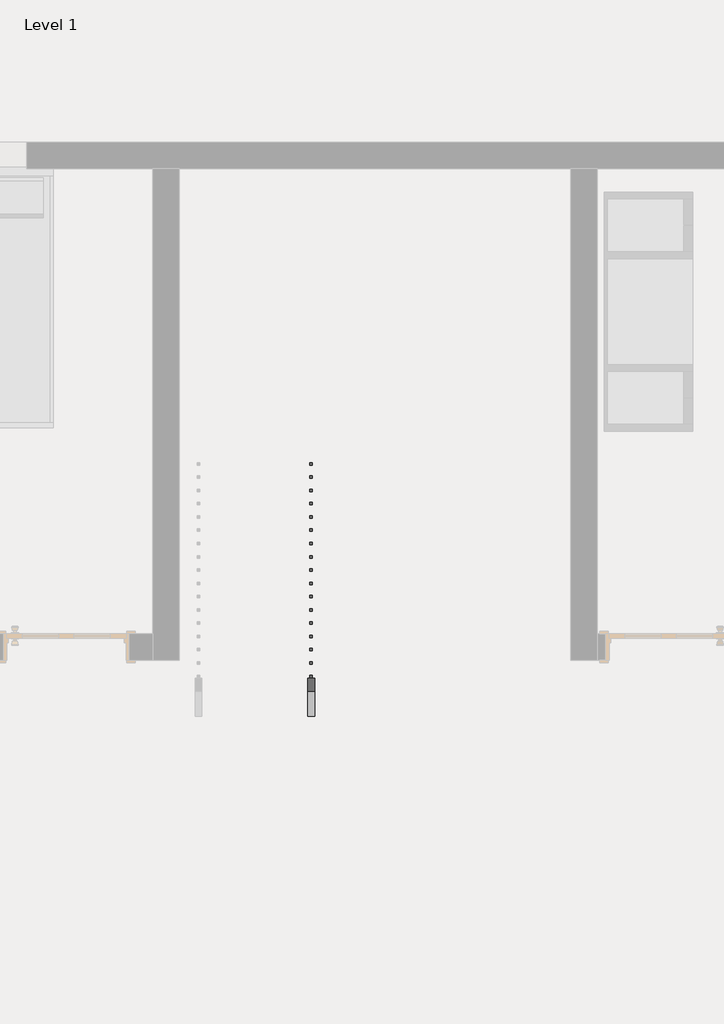
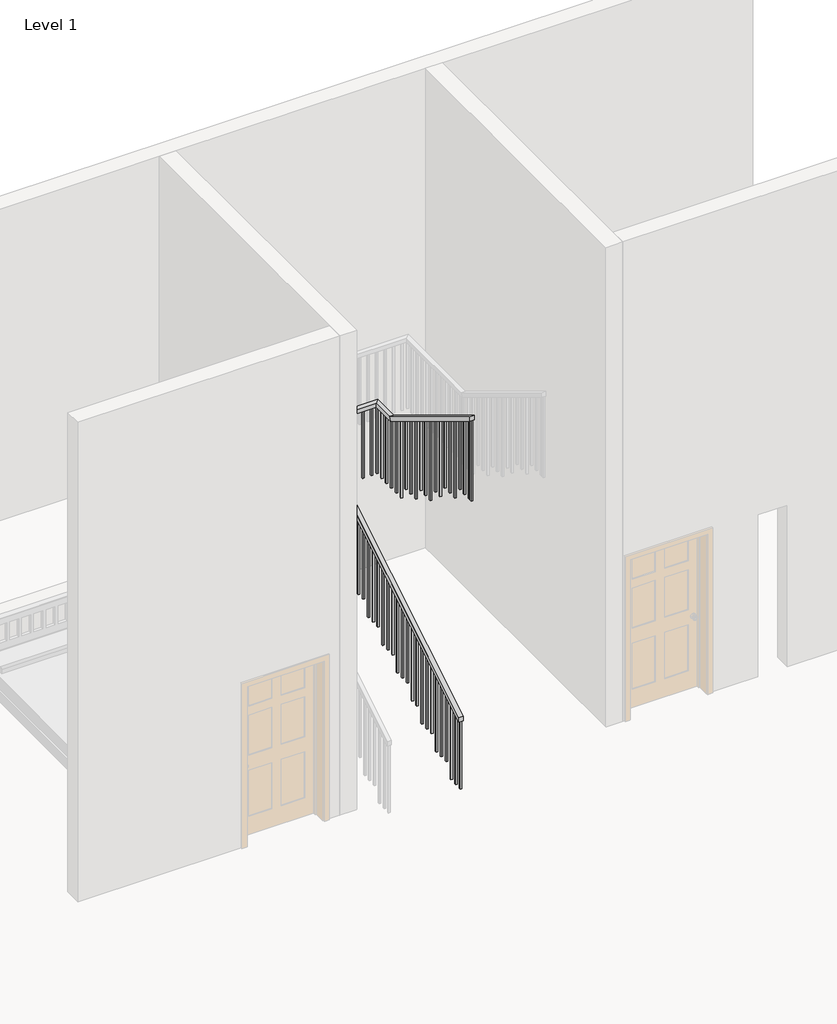
# One storey, part 2 of 3: 1 railing.
"""IFC4 building model written with IfcOpenShell, lengths in millimetres."""

from ifc_helpers import new_model, si_unit, frame, origin, place, context, project, spatial, polyline, outline, extrude, faceted_brep, element, save

model = new_model("IFC4")

# Units and contexts
model_context = context("Model", 3, world=origin())
ifc_project = project(units=[si_unit("LENGTHUNIT", "METRE", prefix="MILLI")], contexts=[model_context])

# Site, building, storey
site = spatial("IfcSite", under=ifc_project)
building = spatial("IfcBuilding", under=site)
storey = spatial("IfcBuildingStorey", under=building, Name="Level 1", Elevation=0.0)

# Railing
placement = place(None, origin())
element("IfcRailing", 1, ObjectType="Handrail - Rectangular", at=placement, inside=storey, context=model_context, shape_type="SolidModel", body=[
    faceted_brep([(-7356.0582637, 8478.2414332, 1083.7333333), (-7356.0582637, 8478.2414332, 1024.3318731), (-7305.2582637, 8478.2414332, 1024.3318731), (-7305.2582637, 8478.2414332, 1083.7333333), (-7356.0582637, 11475.4414332, 2900.2181818), (-7356.0582637, 11526.2414332, 2871.6046004), (-7305.2582637, 11526.2414332, 2871.6046004), (-7305.2582637, 11475.4414332, 2900.2181818), (-7356.0582637, 11475.4414332, 2946.4), (-7356.0582637, 11526.2414332, 2895.6), (-7305.2582637, 11526.2414332, 2895.6), (-7305.2582637, 11475.4414332, 2946.4), (-7356.0582637, 11602.4414332, 2946.4), (-7356.0582637, 11602.4414332, 2895.6), (-7305.2582637, 11551.6414332, 2895.6), (-7305.2582637, 11551.6414332, 2946.4), (-7229.0582637, 11602.4414332, 2946.4), (-7229.0582637, 11602.4414332, 2895.6), (-7229.0582637, 11551.6414332, 2895.6), (-7229.0582637, 11551.6414332, 2946.4), (-6528.1029886, 11602.4414332, 2946.4), (-6528.1029886, 11602.4414332, 2895.6), (-6578.9029886, 11551.6414332, 2895.6), (-6578.9029886, 11551.6414332, 2946.4), (-6528.1029886, 11272.2414332, 2946.4), (-6528.1029886, 11258.0490238, 2895.6), (-6578.9029886, 11258.0490238, 2895.6), (-6578.9029886, 11272.2414332, 2946.4), (-6528.1029886, 9595.8414332, 3962.4), (-6578.9029886, 9595.8414332, 3962.4), (-6578.9029886, 9595.8414332, 3902.9985397), (-6528.1029886, 9595.8414332, 3902.9985397)], [[[0, 1, 2, 3]], [[1, 0, 4, 5]], [[2, 1, 5, 6]], [[3, 2, 6, 7]], [[0, 3, 7, 4]], [[5, 4, 8, 9]], [[6, 5, 9, 10]], [[7, 6, 10, 11]], [[4, 7, 11, 8]], [[9, 8, 12, 13]], [[10, 9, 13, 14]], [[11, 10, 14, 15]], [[8, 11, 15, 12]], [[13, 12, 16, 17]], [[14, 13, 17, 18]], [[15, 14, 18, 19]], [[12, 15, 19, 16]], [[17, 16, 20, 21]], [[18, 17, 21, 22]], [[19, 18, 22, 23]], [[16, 19, 23, 20]], [[21, 20, 24, 25]], [[22, 21, 25, 26]], [[23, 22, 26, 27]], [[20, 23, 27, 24]], [[28, 29, 30, 31]], [[25, 24, 28, 31]], [[26, 25, 31, 30]], [[27, 26, 30, 29]], [[24, 27, 29, 28]]]),
    extrude(outline(polyline([(9637.1164332, 3877.9833882), (9656.1664332, 3866.4379337), (9656.1664332, 2878.6666667), (9637.1164332, 2878.6666667), (9637.1164332, 3877.9833882)])), frame((-6563.0279886, 0.0, 0.0), z_axis=(1.0, 0.0, 0.0), x_axis=(0.0, 1.0, 0.0)), (0.0, 0.0, 1.0), 19.05),
    extrude(outline(polyline([(9738.7164332, 3816.4076307), (9757.7664332, 3804.8621761), (9757.7664332, 2878.6666667), (9738.7164332, 2878.6666667), (9738.7164332, 3816.4076307)])), frame((-6563.0279886, 0.0, 0.0), z_axis=(1.0, 0.0, 0.0), x_axis=(0.0, 1.0, 0.0)), (0.0, 0.0, 1.0), 19.05),
    extrude(outline(polyline([(9840.3164332, 3754.8318731), (9859.3664332, 3743.2864185), (9859.3664332, 2878.6666667), (9840.3164332, 2878.6666667), (9840.3164332, 3754.8318731)])), frame((-6563.0279886, 0.0, 0.0), z_axis=(1.0, 0.0, 0.0), x_axis=(0.0, 1.0, 0.0)), (0.0, 0.0, 1.0), 19.05),
    extrude(outline(polyline([(9941.9164332, 3693.2561155), (9960.9664332, 3681.710661), (9960.9664332, 2709.3333333), (9941.9164332, 2709.3333333), (9941.9164332, 3693.2561155)])), frame((-6563.0279886, 0.0, 0.0), z_axis=(1.0, 0.0, 0.0), x_axis=(0.0, 1.0, 0.0)), (0.0, 0.0, 1.0), 19.05),
    extrude(outline(polyline([(10043.5164332, 3631.6803579), (10062.5664332, 3620.1349034), (10062.5664332, 2709.3333333), (10043.5164332, 2709.3333333), (10043.5164332, 3631.6803579)])), frame((-6563.0279886, 0.0, 0.0), z_axis=(1.0, 0.0, 0.0), x_axis=(0.0, 1.0, 0.0)), (0.0, 0.0, 1.0), 19.05),
    extrude(outline(polyline([(10145.1164332, 3570.1046004), (10164.1664332, 3558.5591458), (10164.1664332, 2709.3333333), (10145.1164332, 2709.3333333), (10145.1164332, 3570.1046004)])), frame((-6563.0279886, 0.0, 0.0), z_axis=(1.0, 0.0, 0.0), x_axis=(0.0, 1.0, 0.0)), (0.0, 0.0, 1.0), 19.05),
    extrude(outline(polyline([(10246.7164332, 3508.5288428), (10265.7664332, 3496.9833882), (10265.7664332, 2540.0), (10246.7164332, 2540.0), (10246.7164332, 3508.5288428)])), frame((-6563.0279886, 0.0, 0.0), z_axis=(1.0, 0.0, 0.0), x_axis=(0.0, 1.0, 0.0)), (0.0, 0.0, 1.0), 19.05),
    extrude(outline(polyline([(10348.3164332, 3446.9530852), (10367.3664332, 3435.4076307), (10367.3664332, 2540.0), (10348.3164332, 2540.0), (10348.3164332, 3446.9530852)])), frame((-6563.0279886, 0.0, 0.0), z_axis=(1.0, 0.0, 0.0), x_axis=(0.0, 1.0, 0.0)), (0.0, 0.0, 1.0), 19.05),
    extrude(outline(polyline([(10449.9164332, 3385.3773276), (10468.9664332, 3373.8318731), (10468.9664332, 2370.6666667), (10449.9164332, 2370.6666667), (10449.9164332, 3385.3773276)])), frame((-6563.0279886, 0.0, 0.0), z_axis=(1.0, 0.0, 0.0), x_axis=(0.0, 1.0, 0.0)), (0.0, 0.0, 1.0), 19.05),
    extrude(outline(polyline([(10551.5164332, 3323.80157), (10570.5664332, 3312.2561155), (10570.5664332, 2370.6666667), (10551.5164332, 2370.6666667), (10551.5164332, 3323.80157)])), frame((-6563.0279886, 0.0, 0.0), z_axis=(1.0, 0.0, 0.0), x_axis=(0.0, 1.0, 0.0)), (0.0, 0.0, 1.0), 19.05),
    extrude(outline(polyline([(10653.1164332, 3262.2258125), (10672.1664332, 3250.6803579), (10672.1664332, 2370.6666667), (10653.1164332, 2370.6666667), (10653.1164332, 3262.2258125)])), frame((-6563.0279886, 0.0, 0.0), z_axis=(1.0, 0.0, 0.0), x_axis=(0.0, 1.0, 0.0)), (0.0, 0.0, 1.0), 19.05),
    extrude(outline(polyline([(10754.7164332, 3200.6500549), (10773.7664332, 3189.1046004), (10773.7664332, 2201.3333333), (10754.7164332, 2201.3333333), (10754.7164332, 3200.6500549)])), frame((-6563.0279886, 0.0, 0.0), z_axis=(1.0, 0.0, 0.0), x_axis=(0.0, 1.0, 0.0)), (0.0, 0.0, 1.0), 19.05),
    extrude(outline(polyline([(10856.3164332, 3139.0742973), (10875.3664332, 3127.5288428), (10875.3664332, 2201.3333333), (10856.3164332, 2201.3333333), (10856.3164332, 3139.0742973)])), frame((-6563.0279886, 0.0, 0.0), z_axis=(1.0, 0.0, 0.0), x_axis=(0.0, 1.0, 0.0)), (0.0, 0.0, 1.0), 19.05),
    extrude(outline(polyline([(10957.9164332, 3077.4985397), (10976.9664332, 3065.9530852), (10976.9664332, 2201.3333333), (10957.9164332, 2201.3333333), (10957.9164332, 3077.4985397)])), frame((-6563.0279886, 0.0, 0.0), z_axis=(1.0, 0.0, 0.0), x_axis=(0.0, 1.0, 0.0)), (0.0, 0.0, 1.0), 19.05),
    extrude(outline(polyline([(11059.5164332, 3015.9227822), (11078.5664332, 3004.3773276), (11078.5664332, 2032.0), (11059.5164332, 2032.0), (11059.5164332, 3015.9227822)])), frame((-6563.0279886, 0.0, 0.0), z_axis=(1.0, 0.0, 0.0), x_axis=(0.0, 1.0, 0.0)), (0.0, 0.0, 1.0), 19.05),
    extrude(outline(polyline([(11161.1164332, 2954.3470246), (11180.1664332, 2942.80157), (11180.1664332, 2032.0), (11161.1164332, 2032.0), (11161.1164332, 2954.3470246)])), frame((-6563.0279886, 0.0, 0.0), z_axis=(1.0, 0.0, 0.0), x_axis=(0.0, 1.0, 0.0)), (0.0, 0.0, 1.0), 19.05),
    extrude(outline(polyline([(-6563.0279886, 11383.3664332), (-6543.9779886, 11383.3664332), (-6543.9779886, 11364.3164332), (-6563.0279886, 11364.3164332), (-6563.0279886, 11383.3664332)])), frame((0.0, 0.0, 2032.0), z_axis=(0.0, 0.0, 1.0), x_axis=(1.0, 0.0, 0.0)), (0.0, 0.0, 1.0), 863.6),
    extrude(outline(polyline([(-6563.0279886, 11484.9664332), (-6543.9779886, 11484.9664332), (-6543.9779886, 11465.9164332), (-6563.0279886, 11465.9164332), (-6563.0279886, 11484.9664332)])), frame((0.0, 0.0, 2032.0), z_axis=(0.0, 0.0, 1.0), x_axis=(1.0, 0.0, 0.0)), (0.0, 0.0, 1.0), 863.6),
    extrude(outline(polyline([(-6628.9832637, 11567.5164332), (-6628.9832637, 11586.5664332), (-6609.9332637, 11586.5664332), (-6609.9332637, 11567.5164332), (-6628.9832637, 11567.5164332)])), frame((0.0, 0.0, 2032.0), z_axis=(0.0, 0.0, 1.0), x_axis=(1.0, 0.0, 0.0)), (0.0, 0.0, 1.0), 863.6),
    extrude(outline(polyline([(-6730.5832637, 11567.5164332), (-6730.5832637, 11586.5664332), (-6711.5332637, 11586.5664332), (-6711.5332637, 11567.5164332), (-6730.5832637, 11567.5164332)])), frame((0.0, 0.0, 2032.0), z_axis=(0.0, 0.0, 1.0), x_axis=(1.0, 0.0, 0.0)), (0.0, 0.0, 1.0), 863.6),
    extrude(outline(polyline([(-6832.1832637, 11567.5164332), (-6832.1832637, 11586.5664332), (-6813.1332637, 11586.5664332), (-6813.1332637, 11567.5164332), (-6832.1832637, 11567.5164332)])), frame((0.0, 0.0, 2032.0), z_axis=(0.0, 0.0, 1.0), x_axis=(1.0, 0.0, 0.0)), (0.0, 0.0, 1.0), 863.6),
    extrude(outline(polyline([(-6933.7832637, 11567.5164332), (-6933.7832637, 11586.5664332), (-6914.7332637, 11586.5664332), (-6914.7332637, 11567.5164332), (-6933.7832637, 11567.5164332)])), frame((0.0, 0.0, 2032.0), z_axis=(0.0, 0.0, 1.0), x_axis=(1.0, 0.0, 0.0)), (0.0, 0.0, 1.0), 863.6),
    extrude(outline(polyline([(-7035.3832637, 11567.5164332), (-7035.3832637, 11586.5664332), (-7016.3332637, 11586.5664332), (-7016.3332637, 11567.5164332), (-7035.3832637, 11567.5164332)])), frame((0.0, 0.0, 2032.0), z_axis=(0.0, 0.0, 1.0), x_axis=(1.0, 0.0, 0.0)), (0.0, 0.0, 1.0), 863.6),
    extrude(outline(polyline([(-7136.9832637, 11567.5164332), (-7136.9832637, 11586.5664332), (-7117.9332637, 11586.5664332), (-7117.9332637, 11567.5164332), (-7136.9832637, 11567.5164332)])), frame((0.0, 0.0, 2032.0), z_axis=(0.0, 0.0, 1.0), x_axis=(1.0, 0.0, 0.0)), (0.0, 0.0, 1.0), 863.6),
    extrude(outline(polyline([(-7238.5832637, 11567.5164332), (-7238.5832637, 11586.5664332), (-7219.5332637, 11586.5664332), (-7219.5332637, 11567.5164332), (-7238.5832637, 11567.5164332)])), frame((0.0, 0.0, 2032.0), z_axis=(0.0, 0.0, 1.0), x_axis=(1.0, 0.0, 0.0)), (0.0, 0.0, 1.0), 863.6),
    extrude(outline(polyline([(11516.7164332, 2865.8318731), (11535.7664332, 2877.3773276), (11535.7664332, 1862.6666667), (11516.7164332, 1862.6666667), (11516.7164332, 2865.8318731)])), frame((-7340.1832637, 0.0, 0.0), z_axis=(1.0, 0.0, 0.0), x_axis=(0.0, 1.0, 0.0)), (0.0, 0.0, 1.0), 19.05),
    extrude(outline(polyline([(11415.1164332, 2804.2561155), (11434.1664332, 2815.80157), (11434.1664332, 1862.6666667), (11415.1164332, 1862.6666667), (11415.1164332, 2804.2561155)])), frame((-7340.1832637, 0.0, 0.0), z_axis=(1.0, 0.0, 0.0), x_axis=(0.0, 1.0, 0.0)), (0.0, 0.0, 1.0), 19.05),
    extrude(outline(polyline([(11313.5164332, 2742.6803579), (11332.5664332, 2754.2258125), (11332.5664332, 1862.6666667), (11313.5164332, 1862.6666667), (11313.5164332, 2742.6803579)])), frame((-7340.1832637, 0.0, 0.0), z_axis=(1.0, 0.0, 0.0), x_axis=(0.0, 1.0, 0.0)), (0.0, 0.0, 1.0), 19.05),
    extrude(outline(polyline([(11211.9164332, 2681.1046004), (11230.9664332, 2692.6500549), (11230.9664332, 1693.3333333), (11211.9164332, 1693.3333333), (11211.9164332, 2681.1046004)])), frame((-7340.1832637, 0.0, 0.0), z_axis=(1.0, 0.0, 0.0), x_axis=(0.0, 1.0, 0.0)), (0.0, 0.0, 1.0), 19.05),
    extrude(outline(polyline([(11110.3164332, 2619.5288428), (11129.3664332, 2631.0742973), (11129.3664332, 1693.3333333), (11110.3164332, 1693.3333333), (11110.3164332, 2619.5288428)])), frame((-7340.1832637, 0.0, 0.0), z_axis=(1.0, 0.0, 0.0), x_axis=(0.0, 1.0, 0.0)), (0.0, 0.0, 1.0), 19.05),
    extrude(outline(polyline([(11008.7164332, 2557.9530852), (11027.7664332, 2569.4985397), (11027.7664332, 1693.3333333), (11008.7164332, 1693.3333333), (11008.7164332, 2557.9530852)])), frame((-7340.1832637, 0.0, 0.0), z_axis=(1.0, 0.0, 0.0), x_axis=(0.0, 1.0, 0.0)), (0.0, 0.0, 1.0), 19.05),
    extrude(outline(polyline([(10907.1164332, 2496.3773276), (10926.1664332, 2507.9227822), (10926.1664332, 1524.0), (10907.1164332, 1524.0), (10907.1164332, 2496.3773276)])), frame((-7340.1832637, 0.0, 0.0), z_axis=(1.0, 0.0, 0.0), x_axis=(0.0, 1.0, 0.0)), (0.0, 0.0, 1.0), 19.05),
    extrude(outline(polyline([(10805.5164332, 2434.80157), (10824.5664332, 2446.3470246), (10824.5664332, 1524.0), (10805.5164332, 1524.0), (10805.5164332, 2434.80157)])), frame((-7340.1832637, 0.0, 0.0), z_axis=(1.0, 0.0, 0.0), x_axis=(0.0, 1.0, 0.0)), (0.0, 0.0, 1.0), 19.05),
    extrude(outline(polyline([(10703.9164332, 2373.2258125), (10722.9664332, 2384.771267), (10722.9664332, 1524.0), (10703.9164332, 1524.0), (10703.9164332, 2373.2258125)])), frame((-7340.1832637, 0.0, 0.0), z_axis=(1.0, 0.0, 0.0), x_axis=(0.0, 1.0, 0.0)), (0.0, 0.0, 1.0), 19.05),
    extrude(outline(polyline([(10602.3164332, 2311.6500549), (10621.3664332, 2323.1955094), (10621.3664332, 1354.6666667), (10602.3164332, 1354.6666667), (10602.3164332, 2311.6500549)])), frame((-7340.1832637, 0.0, 0.0), z_axis=(1.0, 0.0, 0.0), x_axis=(0.0, 1.0, 0.0)), (0.0, 0.0, 1.0), 19.05),
    extrude(outline(polyline([(10500.7164332, 2250.0742973), (10519.7664332, 2261.6197519), (10519.7664332, 1354.6666667), (10500.7164332, 1354.6666667), (10500.7164332, 2250.0742973)])), frame((-7340.1832637, 0.0, 0.0), z_axis=(1.0, 0.0, 0.0), x_axis=(0.0, 1.0, 0.0)), (0.0, 0.0, 1.0), 19.05),
    extrude(outline(polyline([(10399.1164332, 2188.4985397), (10418.1664332, 2200.0439943), (10418.1664332, 1185.3333333), (10399.1164332, 1185.3333333), (10399.1164332, 2188.4985397)])), frame((-7340.1832637, 0.0, 0.0), z_axis=(1.0, 0.0, 0.0), x_axis=(0.0, 1.0, 0.0)), (0.0, 0.0, 1.0), 19.05),
    extrude(outline(polyline([(10297.5164332, 2126.9227822), (10316.5664332, 2138.4682367), (10316.5664332, 1185.3333333), (10297.5164332, 1185.3333333), (10297.5164332, 2126.9227822)])), frame((-7340.1832637, 0.0, 0.0), z_axis=(1.0, 0.0, 0.0), x_axis=(0.0, 1.0, 0.0)), (0.0, 0.0, 1.0), 19.05),
    extrude(outline(polyline([(10195.9164332, 2065.3470246), (10214.9664332, 2076.8924791), (10214.9664332, 1185.3333333), (10195.9164332, 1185.3333333), (10195.9164332, 2065.3470246)])), frame((-7340.1832637, 0.0, 0.0), z_axis=(1.0, 0.0, 0.0), x_axis=(0.0, 1.0, 0.0)), (0.0, 0.0, 1.0), 19.05),
    extrude(outline(polyline([(10094.3164332, 2003.771267), (10113.3664332, 2015.3167216), (10113.3664332, 1016.0), (10094.3164332, 1016.0), (10094.3164332, 2003.771267)])), frame((-7340.1832637, 0.0, 0.0), z_axis=(1.0, 0.0, 0.0), x_axis=(0.0, 1.0, 0.0)), (0.0, 0.0, 1.0), 19.05),
    extrude(outline(polyline([(9992.7164332, 1942.1955094), (10011.7664332, 1953.740964), (10011.7664332, 1016.0), (9992.7164332, 1016.0), (9992.7164332, 1942.1955094)])), frame((-7340.1832637, 0.0, 0.0), z_axis=(1.0, 0.0, 0.0), x_axis=(0.0, 1.0, 0.0)), (0.0, 0.0, 1.0), 19.05),
    extrude(outline(polyline([(9891.1164332, 1880.6197519), (9910.1664332, 1892.1652064), (9910.1664332, 1016.0), (9891.1164332, 1016.0), (9891.1164332, 1880.6197519)])), frame((-7340.1832637, 0.0, 0.0), z_axis=(1.0, 0.0, 0.0), x_axis=(0.0, 1.0, 0.0)), (0.0, 0.0, 1.0), 19.05),
    extrude(outline(polyline([(9789.5164332, 1819.0439943), (9808.5664332, 1830.5894488), (9808.5664332, 846.6666667), (9789.5164332, 846.6666667), (9789.5164332, 1819.0439943)])), frame((-7340.1832637, 0.0, 0.0), z_axis=(1.0, 0.0, 0.0), x_axis=(0.0, 1.0, 0.0)), (0.0, 0.0, 1.0), 19.05),
    extrude(outline(polyline([(9687.9164332, 1757.4682367), (9706.9664332, 1769.0136913), (9706.9664332, 846.6666667), (9687.9164332, 846.6666667), (9687.9164332, 1757.4682367)])), frame((-7340.1832637, 0.0, 0.0), z_axis=(1.0, 0.0, 0.0), x_axis=(0.0, 1.0, 0.0)), (0.0, 0.0, 1.0), 19.05),
    extrude(outline(polyline([(9586.3164332, 1695.8924791), (9605.3664332, 1707.4379337), (9605.3664332, 846.6666667), (9586.3164332, 846.6666667), (9586.3164332, 1695.8924791)])), frame((-7340.1832637, 0.0, 0.0), z_axis=(1.0, 0.0, 0.0), x_axis=(0.0, 1.0, 0.0)), (0.0, 0.0, 1.0), 19.05),
    extrude(outline(polyline([(9484.7164332, 1634.3167216), (9503.7664332, 1645.8621761), (9503.7664332, 677.3333333), (9484.7164332, 677.3333333), (9484.7164332, 1634.3167216)])), frame((-7340.1832637, 0.0, 0.0), z_axis=(1.0, 0.0, 0.0), x_axis=(0.0, 1.0, 0.0)), (0.0, 0.0, 1.0), 19.05),
    extrude(outline(polyline([(9383.1164332, 1572.740964), (9402.1664332, 1584.2864185), (9402.1664332, 677.3333333), (9383.1164332, 677.3333333), (9383.1164332, 1572.740964)])), frame((-7340.1832637, 0.0, 0.0), z_axis=(1.0, 0.0, 0.0), x_axis=(0.0, 1.0, 0.0)), (0.0, 0.0, 1.0), 19.05),
    extrude(outline(polyline([(9281.5164332, 1511.1652064), (9300.5664332, 1522.710661), (9300.5664332, 508.0), (9281.5164332, 508.0), (9281.5164332, 1511.1652064)])), frame((-7340.1832637, 0.0, 0.0), z_axis=(1.0, 0.0, 0.0), x_axis=(0.0, 1.0, 0.0)), (0.0, 0.0, 1.0), 19.05),
    extrude(outline(polyline([(9179.9164332, 1449.5894488), (9198.9664332, 1461.1349034), (9198.9664332, 508.0), (9179.9164332, 508.0), (9179.9164332, 1449.5894488)])), frame((-7340.1832637, 0.0, 0.0), z_axis=(1.0, 0.0, 0.0), x_axis=(0.0, 1.0, 0.0)), (0.0, 0.0, 1.0), 19.05),
    extrude(outline(polyline([(9078.3164332, 1388.0136913), (9097.3664332, 1399.5591458), (9097.3664332, 508.0), (9078.3164332, 508.0), (9078.3164332, 1388.0136913)])), frame((-7340.1832637, 0.0, 0.0), z_axis=(1.0, 0.0, 0.0), x_axis=(0.0, 1.0, 0.0)), (0.0, 0.0, 1.0), 19.05),
    extrude(outline(polyline([(8976.7164332, 1326.4379337), (8995.7664332, 1337.9833882), (8995.7664332, 338.6666667), (8976.7164332, 338.6666667), (8976.7164332, 1326.4379337)])), frame((-7340.1832637, 0.0, 0.0), z_axis=(1.0, 0.0, 0.0), x_axis=(0.0, 1.0, 0.0)), (0.0, 0.0, 1.0), 19.05),
    extrude(outline(polyline([(8875.1164332, 1264.8621761), (8894.1664332, 1276.4076307), (8894.1664332, 338.6666667), (8875.1164332, 338.6666667), (8875.1164332, 1264.8621761)])), frame((-7340.1832637, 0.0, 0.0), z_axis=(1.0, 0.0, 0.0), x_axis=(0.0, 1.0, 0.0)), (0.0, 0.0, 1.0), 19.05),
    extrude(outline(polyline([(8773.5164332, 1203.2864185), (8792.5664332, 1214.8318731), (8792.5664332, 338.6666667), (8773.5164332, 338.6666667), (8773.5164332, 1203.2864185)])), frame((-7340.1832637, 0.0, 0.0), z_axis=(1.0, 0.0, 0.0), x_axis=(0.0, 1.0, 0.0)), (0.0, 0.0, 1.0), 19.05),
    extrude(outline(polyline([(8671.9164332, 1141.710661), (8690.9664332, 1153.2561155), (8690.9664332, 169.3333333), (8671.9164332, 169.3333333), (8671.9164332, 1141.710661)])), frame((-7340.1832637, 0.0, 0.0), z_axis=(1.0, 0.0, 0.0), x_axis=(0.0, 1.0, 0.0)), (0.0, 0.0, 1.0), 19.05),
    extrude(outline(polyline([(8570.3164332, 1080.1349034), (8589.3664332, 1091.6803579), (8589.3664332, 169.3333333), (8570.3164332, 169.3333333), (8570.3164332, 1080.1349034)])), frame((-7340.1832637, 0.0, 0.0), z_axis=(1.0, 0.0, 0.0), x_axis=(0.0, 1.0, 0.0)), (0.0, 0.0, 1.0), 19.05),
    extrude(outline(polyline([(-6563.0279886, 11281.7664332), (-6543.9779886, 11281.7664332), (-6543.9779886, 11262.7164332), (-6563.0279886, 11262.7164332), (-6563.0279886, 11281.7664332)])), frame((0.0, 0.0, 2032.0), z_axis=(0.0, 0.0, 1.0), x_axis=(1.0, 0.0, 0.0)), (0.0, 0.0, 1.0), 863.6),
    extrude(outline(polyline([(-6563.0279886, 11586.5664332), (-6543.9779886, 11586.5664332), (-6543.9779886, 11567.5164332), (-6563.0279886, 11567.5164332), (-6563.0279886, 11586.5664332)])), frame((0.0, 0.0, 2032.0), z_axis=(0.0, 0.0, 1.0), x_axis=(1.0, 0.0, 0.0)), (0.0, 0.0, 1.0), 863.6),
    extrude(outline(polyline([(-7321.1332637, 11567.5164332), (-7340.1832637, 11567.5164332), (-7340.1832637, 11586.5664332), (-7321.1332637, 11586.5664332), (-7321.1332637, 11567.5164332)])), frame((0.0, 0.0, 2032.0), z_axis=(0.0, 0.0, 1.0), x_axis=(1.0, 0.0, 0.0)), (0.0, 0.0, 1.0), 863.6),
    extrude(outline(polyline([(-7321.1332637, 11542.1164332), (-7340.1832637, 11542.1164332), (-7340.1832637, 11561.1664332), (-7321.1332637, 11561.1664332), (-7321.1332637, 11542.1164332)])), frame((0.0, 0.0, 2032.0), z_axis=(0.0, 0.0, 1.0), x_axis=(1.0, 0.0, 0.0)), (0.0, 0.0, 1.0), 863.6),
    extrude(outline(polyline([(9595.8414332, 3902.9985397), (9614.8914332, 3891.4530852), (9614.8914332, 2878.6666667), (9595.8414332, 2878.6666667), (9595.8414332, 3902.9985397)])), frame((-6563.0279886, 0.0, 0.0), z_axis=(1.0, 0.0, 0.0), x_axis=(0.0, 1.0, 0.0)), (0.0, 0.0, 1.0), 19.05),
    extrude(outline(polyline([(8478.2414332, 1024.3318731), (8497.2914332, 1035.8773276), (8497.2914332, 169.3333333), (8478.2414332, 169.3333333), (8478.2414332, 1024.3318731)])), frame((-7340.1832637, 0.0, 0.0), z_axis=(1.0, 0.0, 0.0), x_axis=(0.0, 1.0, 0.0)), (0.0, 0.0, 1.0), 19.05),
])

save(model, "model.ifc")

# Revit data of these elements
# Type "Handrail - Rectangular"
#   Assembly Code = "C2010400"
#   built-in parameter 1008612 = 0.0416667 (stored number, unit not read)
#   built-in parameter 1008611 = 0.0416667 (stored number, unit not read)
#   built-in parameter 1008609 = 0.333333 (stored number, unit not read)
#   built-in parameter 1008604 = 0.166667 (stored number, unit not read)
#   built-in parameter 1008603 = 0.166667 (stored number, unit not read)
#   Railing Height = 3' - 0"
#   built-in parameter 1008630 = 2
#   built-in parameter 1008610 = 2
#   built-in parameter 1008618 = Baluster - Square : 3/4"
# Element 1 (IfcRailing, "Handrail - Rectangular")
#   Phase Created = New Construction
